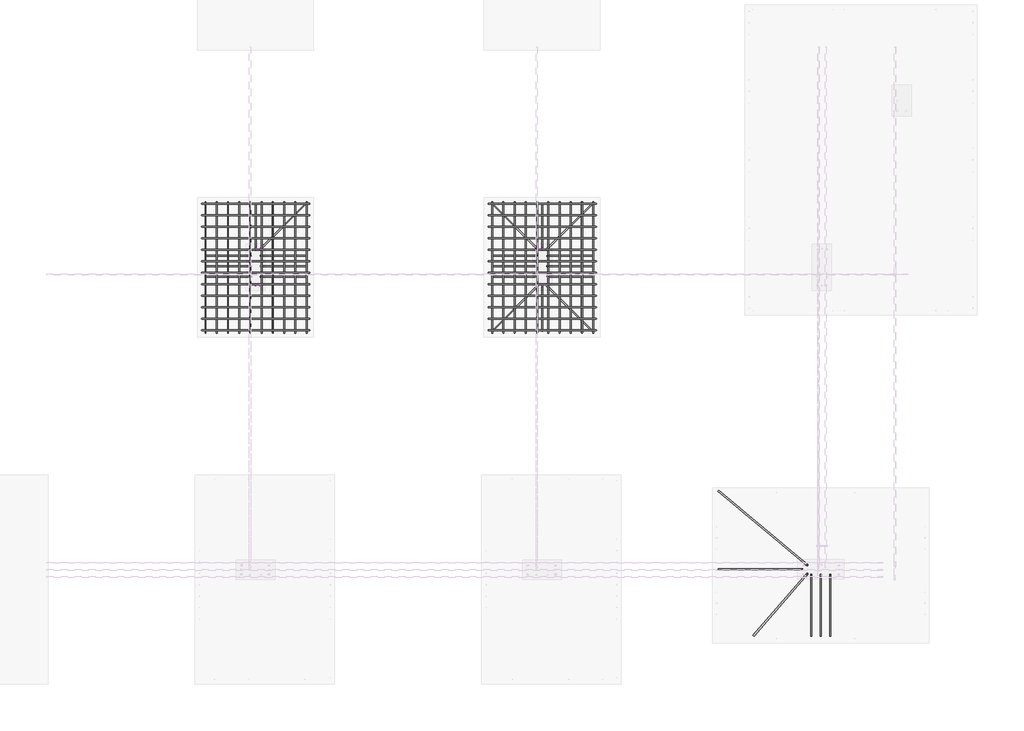
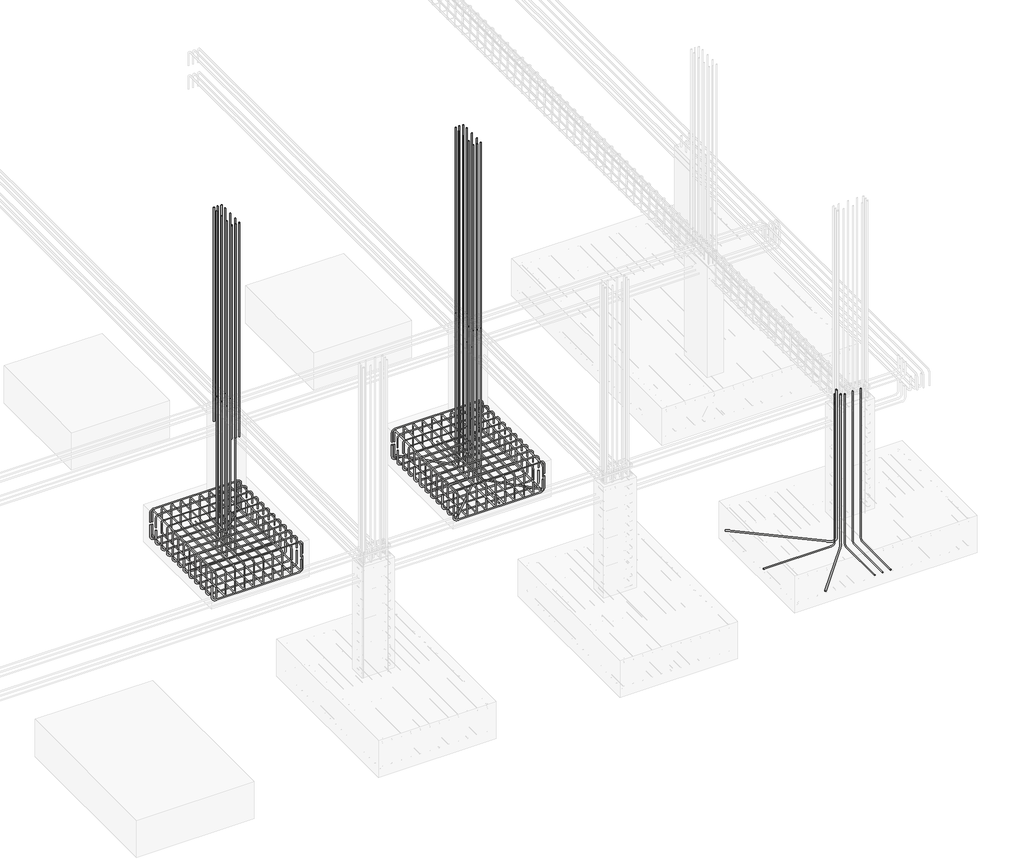
# One storey, part 8 of 18: 40 reinforcing bars.
"""IFC4 building model written with IfcOpenShell, lengths in millimetres."""

from ifc_helpers import new_model, si_unit, point, frame, origin, place, context, project, spatial, polyline, circle_curve, trimmed, segment, composite_curve, source, transform, mapped, element, save
from ifc_brep_helpers import swept_disk

model = new_model("IFC4")

# Units and contexts
model_context = context("Model", 3, world=origin())
ifc_project = project(units=[si_unit("LENGTHUNIT", "METRE", prefix="MILLI")], contexts=[model_context])

# Site, building, storey
site = spatial("IfcSite", under=ifc_project)
building = spatial("IfcBuilding", under=site)
storey = spatial("IfcBuildingStorey", under=building, Elevation=-2000.0)

# Reinforcing bars
placement = place(None, origin())
reinforcing_bar_shape = source(origin(), model_context, "Body", "SolidModel", [
    swept_disk(composite_curve([segment(polyline([(2921.4600308, -834.8555128, -2300.0), (2921.4600308, -834.8555128, -2486.6)]), True, "CONTINUOUS"), segment(trimmed(circle_curve(frame((2866.0100308, -834.8555128, -2486.6), z_axis=(0.0, 1.0, 0.0), x_axis=(55.44999999999982, 0.0, 0.0)), 55.45), [point((2921.4600308, -834.8555128, -2486.6))], [point((2866.0100308, -834.8555128, -2542.05))], True, "CARTESIAN"), True, "CONTINUOUS"), segment(polyline([(2866.0100308, -834.8555128, -2542.05), (1592.8100308, -834.8555128, -2542.05)]), True, "CONTINUOUS"), segment(trimmed(circle_curve(frame((1592.8100308, -834.8555128, -2486.6), z_axis=(0.0, 1.0, 0.0), x_axis=(0.0, 0.0, -55.45000000000027)), 55.45), [point((1592.8100308, -834.8555128, -2542.05))], [point((1537.3600308, -834.8555128, -2486.6))], True, "CARTESIAN"), True, "CONTINUOUS"), segment(polyline([(1537.3600308, -834.8555128, -2486.6), (1537.3600308, -834.8555128, -2300.0)]), True, "CONTINUOUS")], self_intersect=False), 7.95),
])
element("IfcReinforcingBar", 1, at=placement, inside=storey, context=model_context, shape_type="MappedRepresentation", body=[
    mapped(reinforcing_bar_shape, transform((0.0, 0.0, 0.0), x_axis=(1.0, 0.0, 0.0), y_axis=(0.0, 1.0, 0.0), z_axis=(0.0, 0.0, 1.0))),
    mapped(reinforcing_bar_shape, transform((0.0, -148.4250709, 0.0), x_axis=(1.0, 0.0, 0.0), y_axis=(0.0, 1.0, 0.0), z_axis=(0.0, 0.0, 1.0))),
    mapped(reinforcing_bar_shape, transform((0.0, -296.8501418, 0.0), x_axis=(1.0, 0.0, 0.0), y_axis=(0.0, 1.0, 0.0), z_axis=(0.0, 0.0, 1.0))),
    mapped(reinforcing_bar_shape, transform((0.0, -445.2752126, 0.0), x_axis=(1.0, 0.0, 0.0), y_axis=(0.0, 1.0, 0.0), z_axis=(0.0, 0.0, 1.0))),
    mapped(reinforcing_bar_shape, transform((0.0, -593.7002835, 0.0), x_axis=(1.0, 0.0, 0.0), y_axis=(0.0, 1.0, 0.0), z_axis=(0.0, 0.0, 1.0))),
    mapped(reinforcing_bar_shape, transform((0.0, -742.1253544, 0.0), x_axis=(1.0, 0.0, 0.0), y_axis=(0.0, 1.0, 0.0), z_axis=(0.0, 0.0, 1.0))),
    mapped(reinforcing_bar_shape, transform((0.0, -890.5504253, 0.0), x_axis=(1.0, 0.0, 0.0), y_axis=(0.0, 1.0, 0.0), z_axis=(0.0, 0.0, 1.0))),
    mapped(reinforcing_bar_shape, transform((0.0, -1038.9754961, 0.0), x_axis=(1.0, 0.0, 0.0), y_axis=(0.0, 1.0, 0.0), z_axis=(0.0, 0.0, 1.0))),
    mapped(reinforcing_bar_shape, transform((0.0, -1187.400567, 0.0), x_axis=(1.0, 0.0, 0.0), y_axis=(0.0, 1.0, 0.0), z_axis=(0.0, 0.0, 1.0))),
    mapped(reinforcing_bar_shape, transform((0.0, -1335.8256379, 0.0), x_axis=(1.0, 0.0, 0.0), y_axis=(0.0, 1.0, 0.0), z_axis=(0.0, 0.0, 1.0))),
    mapped(reinforcing_bar_shape, transform((0.0, -1484.2507088, 0.0), x_axis=(1.0, 0.0, 0.0), y_axis=(0.0, 1.0, 0.0), z_axis=(0.0, 0.0, 1.0))),
    mapped(reinforcing_bar_shape, transform((0.0, -1632.6757796, 0.0), x_axis=(1.0, 0.0, 0.0), y_axis=(0.0, 1.0, 0.0), z_axis=(0.0, 0.0, 1.0))),
])
reinforcing_bar_2_shape = source(origin(), model_context, "Body", "SolidModel", [
    swept_disk(composite_curve([segment(polyline([(1535.4100308, -834.8555128, -2250.0), (1535.4100308, -834.8555128, -2102.0)]), True, "CONTINUOUS"), segment(trimmed(circle_curve(frame((1581.4100308, -834.8555128, -2102.0), z_axis=(0.0, 1.0, 0.0), x_axis=(-46.0, 0.0, 0.0)), 46.0), [point((1535.4100308, -834.8555128, -2102.0))], [point((1581.4100308, -834.8555128, -2056.0))], True, "CARTESIAN"), True, "CONTINUOUS"), segment(polyline([(1581.4100308, -834.8555128, -2056.0), (2877.4100308, -834.8555128, -2056.0)]), True, "CONTINUOUS"), segment(trimmed(circle_curve(frame((2877.4100308, -834.8555128, -2102.0), z_axis=(0.0, 1.0, 0.0), x_axis=(0.0, 0.0, 46.0)), 46.0), [point((2877.4100308, -834.8555128, -2056.0))], [point((2923.4100308, -834.8555128, -2102.0))], True, "CARTESIAN"), True, "CONTINUOUS"), segment(polyline([(2923.4100308, -834.8555128, -2102.0), (2923.4100308, -834.8555128, -2250.0)]), True, "CONTINUOUS")], self_intersect=False), 6.0),
])
element("IfcReinforcingBar", 2, at=placement, inside=storey, context=model_context, shape_type="MappedRepresentation", body=[
    mapped(reinforcing_bar_2_shape, transform((0.0, 0.0, 0.0), x_axis=(1.0, 0.0, 0.0), y_axis=(0.0, 1.0, 0.0), z_axis=(0.0, 0.0, 1.0))),
    mapped(reinforcing_bar_2_shape, transform((0.0, -148.4250709, 0.0), x_axis=(1.0, 0.0, 0.0), y_axis=(0.0, 1.0, 0.0), z_axis=(0.0, 0.0, 1.0))),
    mapped(reinforcing_bar_2_shape, transform((0.0, -296.8501418, 0.0), x_axis=(1.0, 0.0, 0.0), y_axis=(0.0, 1.0, 0.0), z_axis=(0.0, 0.0, 1.0))),
    mapped(reinforcing_bar_2_shape, transform((0.0, -445.2752126, 0.0), x_axis=(1.0, 0.0, 0.0), y_axis=(0.0, 1.0, 0.0), z_axis=(0.0, 0.0, 1.0))),
    mapped(reinforcing_bar_2_shape, transform((0.0, -593.7002835, 0.0), x_axis=(1.0, 0.0, 0.0), y_axis=(0.0, 1.0, 0.0), z_axis=(0.0, 0.0, 1.0))),
    mapped(reinforcing_bar_2_shape, transform((0.0, -742.1253544, 0.0), x_axis=(1.0, 0.0, 0.0), y_axis=(0.0, 1.0, 0.0), z_axis=(0.0, 0.0, 1.0))),
    mapped(reinforcing_bar_2_shape, transform((0.0, -890.5504253, 0.0), x_axis=(1.0, 0.0, 0.0), y_axis=(0.0, 1.0, 0.0), z_axis=(0.0, 0.0, 1.0))),
    mapped(reinforcing_bar_2_shape, transform((0.0, -1038.9754961, 0.0), x_axis=(1.0, 0.0, 0.0), y_axis=(0.0, 1.0, 0.0), z_axis=(0.0, 0.0, 1.0))),
    mapped(reinforcing_bar_2_shape, transform((0.0, -1187.400567, 0.0), x_axis=(1.0, 0.0, 0.0), y_axis=(0.0, 1.0, 0.0), z_axis=(0.0, 0.0, 1.0))),
    mapped(reinforcing_bar_2_shape, transform((0.0, -1335.8256379, 0.0), x_axis=(1.0, 0.0, 0.0), y_axis=(0.0, 1.0, 0.0), z_axis=(0.0, 0.0, 1.0))),
    mapped(reinforcing_bar_2_shape, transform((0.0, -1484.2507088, 0.0), x_axis=(1.0, 0.0, 0.0), y_axis=(0.0, 1.0, 0.0), z_axis=(0.0, 0.0, 1.0))),
    mapped(reinforcing_bar_2_shape, transform((0.0, -1632.6757796, 0.0), x_axis=(1.0, 0.0, 0.0), y_axis=(0.0, 1.0, 0.0), z_axis=(0.0, 0.0, 1.0))),
])
reinforcing_bar_3_shape = source(origin(), model_context, "Body", "SolidModel", [
    swept_disk(composite_curve([segment(polyline([(1581.5908136, -811.9600376, -2322.6684255), (1581.5908136, -811.9600376, -2470.6684255)]), True, "CONTINUOUS"), segment(trimmed(circle_curve(frame((1581.5908136, -857.9600376, -2470.6684255), z_axis=(-1.0, 0.0, 0.0), x_axis=(0.0, 46.0, 0.0)), 46.0), [point((1581.5908136, -811.9600376, -2470.6684255))], [point((1581.5908136, -857.9600376, -2516.6684255))], True, "CARTESIAN"), True, "CONTINUOUS"), segment(polyline([(1581.5908136, -857.9600376, -2516.6684255), (1581.5908136, -2453.9600376, -2516.6684255)]), True, "CONTINUOUS"), segment(trimmed(circle_curve(frame((1581.5908136, -2453.9600376, -2470.6684255), z_axis=(-1.0, 0.0, 0.0), x_axis=(0.0, 0.0, -46.0)), 46.0), [point((1581.5908136, -2453.9600376, -2516.6684255))], [point((1581.5908136, -2499.9600376, -2470.6684255))], True, "CARTESIAN"), True, "CONTINUOUS"), segment(polyline([(1581.5908136, -2499.9600376, -2470.6684255), (1581.5908136, -2499.9600376, -2322.6684255)]), True, "CONTINUOUS")], self_intersect=False), 6.0),
])
element("IfcReinforcingBar", 3, at=placement, inside=storey, context=model_context, shape_type="MappedRepresentation", body=[
    mapped(reinforcing_bar_3_shape, transform((0.0, 0.0, 0.0), x_axis=(1.0, 0.0, 0.0), y_axis=(0.0, 1.0, 0.0), z_axis=(0.0, 0.0, 1.0))),
    mapped(reinforcing_bar_3_shape, transform((144.8687847, 0.0, 0.0), x_axis=(1.0, 0.0, 0.0), y_axis=(0.0, 1.0, 0.0), z_axis=(0.0, 0.0, 1.0))),
    mapped(reinforcing_bar_3_shape, transform((289.7375694, 0.0, 0.0), x_axis=(1.0, 0.0, 0.0), y_axis=(0.0, 1.0, 0.0), z_axis=(0.0, 0.0, 1.0))),
    mapped(reinforcing_bar_3_shape, transform((434.6063541, 0.0, 0.0), x_axis=(1.0, 0.0, 0.0), y_axis=(0.0, 1.0, 0.0), z_axis=(0.0, 0.0, 1.0))),
    mapped(reinforcing_bar_3_shape, transform((579.4751388, 0.0, 0.0), x_axis=(1.0, 0.0, 0.0), y_axis=(0.0, 1.0, 0.0), z_axis=(0.0, 0.0, 1.0))),
    mapped(reinforcing_bar_3_shape, transform((724.3439235, 0.0, 0.0), x_axis=(1.0, 0.0, 0.0), y_axis=(0.0, 1.0, 0.0), z_axis=(0.0, 0.0, 1.0))),
    mapped(reinforcing_bar_3_shape, transform((869.2127082, 0.0, 0.0), x_axis=(1.0, 0.0, 0.0), y_axis=(0.0, 1.0, 0.0), z_axis=(0.0, 0.0, 1.0))),
    mapped(reinforcing_bar_3_shape, transform((1014.0814929, 0.0, 0.0), x_axis=(1.0, 0.0, 0.0), y_axis=(0.0, 1.0, 0.0), z_axis=(0.0, 0.0, 1.0))),
    mapped(reinforcing_bar_3_shape, transform((1158.9502776, 0.0, 0.0), x_axis=(1.0, 0.0, 0.0), y_axis=(0.0, 1.0, 0.0), z_axis=(0.0, 0.0, 1.0))),
    mapped(reinforcing_bar_3_shape, transform((1303.8190623, 0.0, 0.0), x_axis=(1.0, 0.0, 0.0), y_axis=(0.0, 1.0, 0.0), z_axis=(0.0, 0.0, 1.0))),
])
reinforcing_bar_4_shape = source(origin(), model_context, "Body", "SolidModel", [
    swept_disk(composite_curve([segment(polyline([(2887.3330478, -811.9600376, -2276.6677805), (2887.3330478, -811.9600376, -2128.6677805)]), True, "CONTINUOUS"), segment(trimmed(circle_curve(frame((2887.3330478, -857.9600376, -2128.6677805), z_axis=(1.0, 0.0, 0.0), x_axis=(0.0, 46.0, 0.0)), 46.0), [point((2887.3330478, -811.9600376, -2128.6677805))], [point((2887.3330478, -857.9600376, -2082.6677805))], True, "CARTESIAN"), True, "CONTINUOUS"), segment(polyline([(2887.3330478, -857.9600376, -2082.6677805), (2887.3330478, -2453.9600376, -2082.6677805)]), True, "CONTINUOUS"), segment(trimmed(circle_curve(frame((2887.3330478, -2453.9600376, -2128.6677805), z_axis=(1.0, 0.0, 0.0), x_axis=(0.0, 0.0, 46.0)), 46.0), [point((2887.3330478, -2453.9600376, -2082.6677805))], [point((2887.3330478, -2499.9600376, -2128.6677805))], True, "CARTESIAN"), True, "CONTINUOUS"), segment(polyline([(2887.3330478, -2499.9600376, -2128.6677805), (2887.3330478, -2499.9600376, -2276.6677805)]), True, "CONTINUOUS")], self_intersect=False), 6.0),
])
element("IfcReinforcingBar", 4, at=placement, inside=storey, context=model_context, shape_type="MappedRepresentation", body=[
    mapped(reinforcing_bar_4_shape, transform((0.0, 0.0, 0.0), x_axis=(1.0, 0.0, 0.0), y_axis=(0.0, 1.0, 0.0), z_axis=(0.0, 0.0, 1.0))),
    mapped(reinforcing_bar_4_shape, transform((-145.0824705, 0.0, 0.0), x_axis=(1.0, 0.0, 0.0), y_axis=(0.0, 1.0, 0.0), z_axis=(0.0, 0.0, 1.0))),
    mapped(reinforcing_bar_4_shape, transform((-290.1649409, 0.0, 0.0), x_axis=(1.0, 0.0, 0.0), y_axis=(0.0, 1.0, 0.0), z_axis=(0.0, 0.0, 1.0))),
    mapped(reinforcing_bar_4_shape, transform((-435.2474114, 0.0, 0.0), x_axis=(1.0, 0.0, 0.0), y_axis=(0.0, 1.0, 0.0), z_axis=(0.0, 0.0, 1.0))),
    mapped(reinforcing_bar_4_shape, transform((-580.3298819, 0.0, 0.0), x_axis=(1.0, 0.0, 0.0), y_axis=(0.0, 1.0, 0.0), z_axis=(0.0, 0.0, 1.0))),
    mapped(reinforcing_bar_4_shape, transform((-725.4123523, 0.0, 0.0), x_axis=(1.0, 0.0, 0.0), y_axis=(0.0, 1.0, 0.0), z_axis=(0.0, 0.0, 1.0))),
    mapped(reinforcing_bar_4_shape, transform((-870.4948228, 0.0, 0.0), x_axis=(1.0, 0.0, 0.0), y_axis=(0.0, 1.0, 0.0), z_axis=(0.0, 0.0, 1.0))),
    mapped(reinforcing_bar_4_shape, transform((-1015.5772932, 0.0, 0.0), x_axis=(1.0, 0.0, 0.0), y_axis=(0.0, 1.0, 0.0), z_axis=(0.0, 0.0, 1.0))),
    mapped(reinforcing_bar_4_shape, transform((-1160.6597637, 0.0, 0.0), x_axis=(1.0, 0.0, 0.0), y_axis=(0.0, 1.0, 0.0), z_axis=(0.0, 0.0, 1.0))),
    mapped(reinforcing_bar_4_shape, transform((-1305.7422342, 0.0, 0.0), x_axis=(1.0, 0.0, 0.0), y_axis=(0.0, 1.0, 0.0), z_axis=(0.0, 0.0, 1.0))),
])
reinforcing_bar_5_shape = source(origin(), model_context, "Body", "SolidModel", [
    swept_disk(composite_curve([segment(polyline([(6621.4600308, -834.8555128, -2300.0), (6621.4600308, -834.8555128, -2486.6)]), True, "CONTINUOUS"), segment(trimmed(circle_curve(frame((6566.0100308, -834.8555128, -2486.6), z_axis=(0.0, 1.0, 0.0), x_axis=(55.44999999999982, 0.0, 0.0)), 55.45), [point((6621.4600308, -834.8555128, -2486.6))], [point((6566.0100308, -834.8555128, -2542.05))], True, "CARTESIAN"), True, "CONTINUOUS"), segment(polyline([(6566.0100308, -834.8555128, -2542.05), (5292.8100308, -834.8555128, -2542.05)]), True, "CONTINUOUS"), segment(trimmed(circle_curve(frame((5292.8100308, -834.8555128, -2486.6), z_axis=(0.0, 1.0, 0.0), x_axis=(0.0, 0.0, -55.45000000000027)), 55.45), [point((5292.8100308, -834.8555128, -2542.05))], [point((5237.3600308, -834.8555128, -2486.6))], True, "CARTESIAN"), True, "CONTINUOUS"), segment(polyline([(5237.3600308, -834.8555128, -2486.6), (5237.3600308, -834.8555128, -2300.0)]), True, "CONTINUOUS")], self_intersect=False), 7.95),
])
element("IfcReinforcingBar", 5, at=placement, inside=storey, context=model_context, shape_type="MappedRepresentation", body=[
    mapped(reinforcing_bar_5_shape, transform((0.0, 0.0, 0.0), x_axis=(1.0, 0.0, 0.0), y_axis=(0.0, 1.0, 0.0), z_axis=(0.0, 0.0, 1.0))),
    mapped(reinforcing_bar_5_shape, transform((0.0, -148.4250709, 0.0), x_axis=(1.0, 0.0, 0.0), y_axis=(0.0, 1.0, 0.0), z_axis=(0.0, 0.0, 1.0))),
    mapped(reinforcing_bar_5_shape, transform((0.0, -296.8501418, 0.0), x_axis=(1.0, 0.0, 0.0), y_axis=(0.0, 1.0, 0.0), z_axis=(0.0, 0.0, 1.0))),
    mapped(reinforcing_bar_5_shape, transform((0.0, -445.2752126, 0.0), x_axis=(1.0, 0.0, 0.0), y_axis=(0.0, 1.0, 0.0), z_axis=(0.0, 0.0, 1.0))),
    mapped(reinforcing_bar_5_shape, transform((0.0, -593.7002835, 0.0), x_axis=(1.0, 0.0, 0.0), y_axis=(0.0, 1.0, 0.0), z_axis=(0.0, 0.0, 1.0))),
    mapped(reinforcing_bar_5_shape, transform((0.0, -742.1253544, 0.0), x_axis=(1.0, 0.0, 0.0), y_axis=(0.0, 1.0, 0.0), z_axis=(0.0, 0.0, 1.0))),
    mapped(reinforcing_bar_5_shape, transform((0.0, -890.5504253, 0.0), x_axis=(1.0, 0.0, 0.0), y_axis=(0.0, 1.0, 0.0), z_axis=(0.0, 0.0, 1.0))),
    mapped(reinforcing_bar_5_shape, transform((0.0, -1038.9754961, 0.0), x_axis=(1.0, 0.0, 0.0), y_axis=(0.0, 1.0, 0.0), z_axis=(0.0, 0.0, 1.0))),
    mapped(reinforcing_bar_5_shape, transform((0.0, -1187.400567, 0.0), x_axis=(1.0, 0.0, 0.0), y_axis=(0.0, 1.0, 0.0), z_axis=(0.0, 0.0, 1.0))),
    mapped(reinforcing_bar_5_shape, transform((0.0, -1335.8256379, 0.0), x_axis=(1.0, 0.0, 0.0), y_axis=(0.0, 1.0, 0.0), z_axis=(0.0, 0.0, 1.0))),
    mapped(reinforcing_bar_5_shape, transform((0.0, -1484.2507088, 0.0), x_axis=(1.0, 0.0, 0.0), y_axis=(0.0, 1.0, 0.0), z_axis=(0.0, 0.0, 1.0))),
    mapped(reinforcing_bar_5_shape, transform((0.0, -1632.6757796, 0.0), x_axis=(1.0, 0.0, 0.0), y_axis=(0.0, 1.0, 0.0), z_axis=(0.0, 0.0, 1.0))),
])
reinforcing_bar_6_shape = source(origin(), model_context, "Body", "SolidModel", [
    swept_disk(composite_curve([segment(polyline([(5235.4100308, -834.8555128, -2250.0), (5235.4100308, -834.8555128, -2102.0)]), True, "CONTINUOUS"), segment(trimmed(circle_curve(frame((5281.4100308, -834.8555128, -2102.0), z_axis=(0.0, 1.0, 0.0), x_axis=(-46.0, 0.0, 0.0)), 46.0), [point((5235.4100308, -834.8555128, -2102.0))], [point((5281.4100308, -834.8555128, -2056.0))], True, "CARTESIAN"), True, "CONTINUOUS"), segment(polyline([(5281.4100308, -834.8555128, -2056.0), (6577.4100308, -834.8555128, -2056.0)]), True, "CONTINUOUS"), segment(trimmed(circle_curve(frame((6577.4100308, -834.8555128, -2102.0), z_axis=(0.0, 1.0, 0.0), x_axis=(0.0, 0.0, 46.0)), 46.0), [point((6577.4100308, -834.8555128, -2056.0))], [point((6623.4100308, -834.8555128, -2102.0))], True, "CARTESIAN"), True, "CONTINUOUS"), segment(polyline([(6623.4100308, -834.8555128, -2102.0), (6623.4100308, -834.8555128, -2250.0)]), True, "CONTINUOUS")], self_intersect=False), 6.0),
])
element("IfcReinforcingBar", 6, at=placement, inside=storey, context=model_context, shape_type="MappedRepresentation", body=[
    mapped(reinforcing_bar_6_shape, transform((0.0, 0.0, 0.0), x_axis=(1.0, 0.0, 0.0), y_axis=(0.0, 1.0, 0.0), z_axis=(0.0, 0.0, 1.0))),
    mapped(reinforcing_bar_6_shape, transform((0.0, -148.4250709, 0.0), x_axis=(1.0, 0.0, 0.0), y_axis=(0.0, 1.0, 0.0), z_axis=(0.0, 0.0, 1.0))),
    mapped(reinforcing_bar_6_shape, transform((0.0, -296.8501418, 0.0), x_axis=(1.0, 0.0, 0.0), y_axis=(0.0, 1.0, 0.0), z_axis=(0.0, 0.0, 1.0))),
    mapped(reinforcing_bar_6_shape, transform((0.0, -445.2752126, 0.0), x_axis=(1.0, 0.0, 0.0), y_axis=(0.0, 1.0, 0.0), z_axis=(0.0, 0.0, 1.0))),
    mapped(reinforcing_bar_6_shape, transform((0.0, -593.7002835, 0.0), x_axis=(1.0, 0.0, 0.0), y_axis=(0.0, 1.0, 0.0), z_axis=(0.0, 0.0, 1.0))),
    mapped(reinforcing_bar_6_shape, transform((0.0, -742.1253544, 0.0), x_axis=(1.0, 0.0, 0.0), y_axis=(0.0, 1.0, 0.0), z_axis=(0.0, 0.0, 1.0))),
    mapped(reinforcing_bar_6_shape, transform((0.0, -890.5504253, 0.0), x_axis=(1.0, 0.0, 0.0), y_axis=(0.0, 1.0, 0.0), z_axis=(0.0, 0.0, 1.0))),
    mapped(reinforcing_bar_6_shape, transform((0.0, -1038.9754961, 0.0), x_axis=(1.0, 0.0, 0.0), y_axis=(0.0, 1.0, 0.0), z_axis=(0.0, 0.0, 1.0))),
    mapped(reinforcing_bar_6_shape, transform((0.0, -1187.400567, 0.0), x_axis=(1.0, 0.0, 0.0), y_axis=(0.0, 1.0, 0.0), z_axis=(0.0, 0.0, 1.0))),
    mapped(reinforcing_bar_6_shape, transform((0.0, -1335.8256379, 0.0), x_axis=(1.0, 0.0, 0.0), y_axis=(0.0, 1.0, 0.0), z_axis=(0.0, 0.0, 1.0))),
    mapped(reinforcing_bar_6_shape, transform((0.0, -1484.2507088, 0.0), x_axis=(1.0, 0.0, 0.0), y_axis=(0.0, 1.0, 0.0), z_axis=(0.0, 0.0, 1.0))),
    mapped(reinforcing_bar_6_shape, transform((0.0, -1632.6757796, 0.0), x_axis=(1.0, 0.0, 0.0), y_axis=(0.0, 1.0, 0.0), z_axis=(0.0, 0.0, 1.0))),
])
reinforcing_bar_7_shape = source(origin(), model_context, "Body", "SolidModel", [
    swept_disk(composite_curve([segment(polyline([(5281.5908136, -811.9600376, -2322.6684255), (5281.5908136, -811.9600376, -2470.6684255)]), True, "CONTINUOUS"), segment(trimmed(circle_curve(frame((5281.5908136, -857.9600376, -2470.6684255), z_axis=(-1.0, 0.0, 0.0), x_axis=(0.0, 46.0, 0.0)), 46.0), [point((5281.5908136, -811.9600376, -2470.6684255))], [point((5281.5908136, -857.9600376, -2516.6684255))], True, "CARTESIAN"), True, "CONTINUOUS"), segment(polyline([(5281.5908136, -857.9600376, -2516.6684255), (5281.5908136, -2453.9600376, -2516.6684255)]), True, "CONTINUOUS"), segment(trimmed(circle_curve(frame((5281.5908136, -2453.9600376, -2470.6684255), z_axis=(-1.0, 0.0, 0.0), x_axis=(0.0, 0.0, -46.0)), 46.0), [point((5281.5908136, -2453.9600376, -2516.6684255))], [point((5281.5908136, -2499.9600376, -2470.6684255))], True, "CARTESIAN"), True, "CONTINUOUS"), segment(polyline([(5281.5908136, -2499.9600376, -2470.6684255), (5281.5908136, -2499.9600376, -2322.6684255)]), True, "CONTINUOUS")], self_intersect=False), 6.0),
])
element("IfcReinforcingBar", 7, at=placement, inside=storey, context=model_context, shape_type="MappedRepresentation", body=[
    mapped(reinforcing_bar_7_shape, transform((0.0, 0.0, 0.0), x_axis=(1.0, 0.0, 0.0), y_axis=(0.0, 1.0, 0.0), z_axis=(0.0, 0.0, 1.0))),
    mapped(reinforcing_bar_7_shape, transform((144.8687847, 0.0, 0.0), x_axis=(1.0, 0.0, 0.0), y_axis=(0.0, 1.0, 0.0), z_axis=(0.0, 0.0, 1.0))),
    mapped(reinforcing_bar_7_shape, transform((289.7375694, 0.0, 0.0), x_axis=(1.0, 0.0, 0.0), y_axis=(0.0, 1.0, 0.0), z_axis=(0.0, 0.0, 1.0))),
    mapped(reinforcing_bar_7_shape, transform((434.6063541, 0.0, 0.0), x_axis=(1.0, 0.0, 0.0), y_axis=(0.0, 1.0, 0.0), z_axis=(0.0, 0.0, 1.0))),
    mapped(reinforcing_bar_7_shape, transform((579.4751388, 0.0, 0.0), x_axis=(1.0, 0.0, 0.0), y_axis=(0.0, 1.0, 0.0), z_axis=(0.0, 0.0, 1.0))),
    mapped(reinforcing_bar_7_shape, transform((724.3439235, 0.0, 0.0), x_axis=(1.0, 0.0, 0.0), y_axis=(0.0, 1.0, 0.0), z_axis=(0.0, 0.0, 1.0))),
    mapped(reinforcing_bar_7_shape, transform((869.2127082, 0.0, 0.0), x_axis=(1.0, 0.0, 0.0), y_axis=(0.0, 1.0, 0.0), z_axis=(0.0, 0.0, 1.0))),
    mapped(reinforcing_bar_7_shape, transform((1014.0814929, 0.0, 0.0), x_axis=(1.0, 0.0, 0.0), y_axis=(0.0, 1.0, 0.0), z_axis=(0.0, 0.0, 1.0))),
    mapped(reinforcing_bar_7_shape, transform((1158.9502776, 0.0, 0.0), x_axis=(1.0, 0.0, 0.0), y_axis=(0.0, 1.0, 0.0), z_axis=(0.0, 0.0, 1.0))),
    mapped(reinforcing_bar_7_shape, transform((1303.8190623, 0.0, 0.0), x_axis=(1.0, 0.0, 0.0), y_axis=(0.0, 1.0, 0.0), z_axis=(0.0, 0.0, 1.0))),
])
reinforcing_bar_8_shape = source(origin(), model_context, "Body", "SolidModel", [
    swept_disk(composite_curve([segment(polyline([(6587.3330478, -811.9600376, -2276.6677805), (6587.3330478, -811.9600376, -2128.6677805)]), True, "CONTINUOUS"), segment(trimmed(circle_curve(frame((6587.3330478, -857.9600376, -2128.6677805), z_axis=(1.0, 0.0, 0.0), x_axis=(0.0, 46.0, 0.0)), 46.0), [point((6587.3330478, -811.9600376, -2128.6677805))], [point((6587.3330478, -857.9600376, -2082.6677805))], True, "CARTESIAN"), True, "CONTINUOUS"), segment(polyline([(6587.3330478, -857.9600376, -2082.6677805), (6587.3330478, -2453.9600376, -2082.6677805)]), True, "CONTINUOUS"), segment(trimmed(circle_curve(frame((6587.3330478, -2453.9600376, -2128.6677805), z_axis=(1.0, 0.0, 0.0), x_axis=(0.0, 0.0, 46.0)), 46.0), [point((6587.3330478, -2453.9600376, -2082.6677805))], [point((6587.3330478, -2499.9600376, -2128.6677805))], True, "CARTESIAN"), True, "CONTINUOUS"), segment(polyline([(6587.3330478, -2499.9600376, -2128.6677805), (6587.3330478, -2499.9600376, -2276.6677805)]), True, "CONTINUOUS")], self_intersect=False), 6.0),
])
element("IfcReinforcingBar", 8, at=placement, inside=storey, context=model_context, shape_type="MappedRepresentation", body=[
    mapped(reinforcing_bar_8_shape, transform((0.0, 0.0, 0.0), x_axis=(1.0, 0.0, 0.0), y_axis=(0.0, 1.0, 0.0), z_axis=(0.0, 0.0, 1.0))),
    mapped(reinforcing_bar_8_shape, transform((-145.0824705, 0.0, 0.0), x_axis=(1.0, 0.0, 0.0), y_axis=(0.0, 1.0, 0.0), z_axis=(0.0, 0.0, 1.0))),
    mapped(reinforcing_bar_8_shape, transform((-290.1649409, 0.0, 0.0), x_axis=(1.0, 0.0, 0.0), y_axis=(0.0, 1.0, 0.0), z_axis=(0.0, 0.0, 1.0))),
    mapped(reinforcing_bar_8_shape, transform((-435.2474114, 0.0, 0.0), x_axis=(1.0, 0.0, 0.0), y_axis=(0.0, 1.0, 0.0), z_axis=(0.0, 0.0, 1.0))),
    mapped(reinforcing_bar_8_shape, transform((-580.3298819, 0.0, 0.0), x_axis=(1.0, 0.0, 0.0), y_axis=(0.0, 1.0, 0.0), z_axis=(0.0, 0.0, 1.0))),
    mapped(reinforcing_bar_8_shape, transform((-725.4123523, 0.0, 0.0), x_axis=(1.0, 0.0, 0.0), y_axis=(0.0, 1.0, 0.0), z_axis=(0.0, 0.0, 1.0))),
    mapped(reinforcing_bar_8_shape, transform((-870.4948228, 0.0, 0.0), x_axis=(1.0, 0.0, 0.0), y_axis=(0.0, 1.0, 0.0), z_axis=(0.0, 0.0, 1.0))),
    mapped(reinforcing_bar_8_shape, transform((-1015.5772932, 0.0, 0.0), x_axis=(1.0, 0.0, 0.0), y_axis=(0.0, 1.0, 0.0), z_axis=(0.0, 0.0, 1.0))),
    mapped(reinforcing_bar_8_shape, transform((-1160.6597637, 0.0, 0.0), x_axis=(1.0, 0.0, 0.0), y_axis=(0.0, 1.0, 0.0), z_axis=(0.0, 0.0, 1.0))),
    mapped(reinforcing_bar_8_shape, transform((-1305.7422342, 0.0, 0.0), x_axis=(1.0, 0.0, 0.0), y_axis=(0.0, 1.0, 0.0), z_axis=(0.0, 0.0, 1.0))),
])
element("IfcReinforcingBar", 9, at=placement, inside=storey, context=model_context, shape_type="SolidModel", body=[
    swept_disk(composite_curve([segment(polyline([(8202.5916138, -4537.960597, -2480.0), (9296.0051153, -5455.4434628, -2480.0)]), True, "CONTINUOUS"), segment(trimmed(circle_curve(frame((9296.0051153, -5455.4434628, -2412.5), z_axis=(-0.6427876096865429, -0.766044443118975, 0.0), x_axis=(0.0, 0.0, -67.5)), 67.5), [point((9296.0051153, -5455.4434628, -2480.0))], [point((9347.7131152, -5498.8316264, -2412.5))], True, "CARTESIAN"), True, "CONTINUOUS"), segment(polyline([(9347.7131152, -5498.8316264, -2412.5), (9347.7131152, -5498.8316264, -20.0)]), True, "CONTINUOUS")], self_intersect=False), 10.0),
])
element("IfcReinforcingBar", 10, at=placement, inside=storey, context=model_context, shape_type="SolidModel", body=[
    swept_disk(composite_curve([segment(polyline([(8198.5572946, -5554.0856321, -2480.0), (9241.3529891, -5554.0856321, -2480.0)]), True, "CONTINUOUS"), segment(trimmed(circle_curve(frame((9241.3529891, -5554.0856321, -2434.0), z_axis=(0.0, -1.0, 0.0), x_axis=(0.0, 0.0, -46.0)), 46.0), [point((9241.3529891, -5554.0856321, -2480.0))], [point((9287.3529891, -5554.0856321, -2434.0))], True, "CARTESIAN"), True, "CONTINUOUS"), segment(polyline([(9287.3529891, -5554.0856321, -2434.0), (9287.3529891, -5554.0856321, -30.0)]), True, "CONTINUOUS")], self_intersect=False), 6.0),
])
element("IfcReinforcingBar", 11, at=placement, inside=storey, context=model_context, shape_type="SolidModel", body=[
    swept_disk(composite_curve([segment(polyline([(8655.8433207, -6409.8777562, -2480.0), (9303.4291308, -5664.9154994, -2480.0)]), True, "CONTINUOUS"), segment(trimmed(circle_curve(frame((9303.4291308, -5664.9154994, -2412.5), z_axis=(0.7547095802227678, -0.6560590289905122, 0.0), x_axis=(0.0, 0.0, -67.5)), 67.5), [point((9303.4291308, -5664.9154994, -2480.0))], [point((9347.7131152, -5613.9726027, -2412.5))], True, "CARTESIAN"), True, "CONTINUOUS"), segment(polyline([(9347.7131152, -5613.9726027, -2412.5), (9347.7131152, -5613.9726027, -20.0)]), True, "CONTINUOUS")], self_intersect=False), 10.0),
])
reinforcing_bar_9_shape = source(origin(), model_context, "Body", "SolidModel", [
    swept_disk(composite_curve([segment(polyline([(9402.8188559, -6417.9733694, -2480.0), (9402.8188559, -5668.4399471, -2480.0)]), True, "CONTINUOUS"), segment(trimmed(circle_curve(frame((9402.8188559, -5668.4399471, -2434.0), z_axis=(1.0, 0.0, 0.0), x_axis=(0.0, 0.0, -46.0)), 46.0), [point((9402.8188559, -5668.4399471, -2480.0))], [point((9402.8188559, -5622.4399471, -2434.0))], True, "CARTESIAN"), True, "CONTINUOUS"), segment(polyline([(9402.8188559, -5622.4399471, -2434.0), (9402.8188559, -5622.4399471, -30.0)]), True, "CONTINUOUS")], self_intersect=False), 6.0),
])
element("IfcReinforcingBar", 12, at=placement, inside=storey, context=model_context, shape_type="MappedRepresentation", body=[
    mapped(reinforcing_bar_9_shape, transform((0.0, 0.0, 0.0), x_axis=(1.0, 0.0, 0.0), y_axis=(0.0, 1.0, 0.0), z_axis=(0.0, 0.0, 1.0))),
    mapped(reinforcing_bar_9_shape, transform((122.4797009, 0.0, 0.0), x_axis=(1.0, 0.0, 0.0), y_axis=(0.0, 1.0, 0.0), z_axis=(0.0, 0.0, 1.0))),
    mapped(reinforcing_bar_9_shape, transform((244.9594019, 0.0, 0.0), x_axis=(1.0, 0.0, 0.0), y_axis=(0.0, 1.0, 0.0), z_axis=(0.0, 0.0, 1.0))),
])
element("IfcReinforcingBar", 13, at=placement, inside=storey, context=model_context, shape_type="SolidModel", body=[
    swept_disk(composite_curve([segment(polyline([(5871.6640946, -1423.0839981, -30.0), (5871.6640946, -1423.0839981, -2431.15)]), True, "CONTINUOUS"), segment(trimmed(circle_curve(frame((5832.4550236, -1383.874927, -2431.15), z_axis=(0.70710678118655, 0.707106781186545, 0.0), x_axis=(39.20907100000022, -39.209071099999846, 0.0)), 55.45), [point((5871.6640946, -1423.0839981, -2431.15))], [point((5832.4550236, -1383.874927, -2486.6))], True, "CARTESIAN"), True, "CONTINUOUS"), segment(polyline([(5832.4550236, -1383.874927, -2486.6), (5286.60971, -838.0296134, -2486.6)]), True, "CONTINUOUS")], self_intersect=False), 7.95),
])
element("IfcReinforcingBar", 14, at=placement, inside=storey, context=model_context, shape_type="SolidModel", body=[
    swept_disk(composite_curve([segment(polyline([(5928.962113, -1418.4824597, -30.0), (5928.962113, -1418.4824597, -2440.6)]), True, "CONTINUOUS"), segment(trimmed(circle_curve(frame((5928.962113, -1372.4824597, -2440.6), z_axis=(1.0, 0.0, 0.0), x_axis=(0.0, -46.0, 0.0)), 46.0), [point((5928.962113, -1418.4824597, -2440.6))], [point((5928.962113, -1372.4824597, -2486.6))], True, "CARTESIAN"), True, "CONTINUOUS"), segment(polyline([(5928.962113, -1372.4824597, -2486.6), (5928.962113, -834.8555128, -2486.6)]), True, "CONTINUOUS")], self_intersect=False), 6.0),
])
reinforcing_bar_10_shape = source(origin(), model_context, "Body", "SolidModel", [
    swept_disk(composite_curve([segment(polyline([(5865.503375, -1776.5422299, -30.0), (5865.503375, -1776.5422299, -2436.6982733)]), True, "CONTINUOUS"), segment(trimmed(circle_curve(frame((5819.503375, -1776.5422299, -2436.6982733), z_axis=(0.0, 1.0, 0.0), x_axis=(46.0, 0.0, 0.0)), 46.0), [point((5865.503375, -1776.5422299, -2436.6982733))], [point((5819.503375, -1776.5422299, -2482.6982733))], True, "CARTESIAN"), True, "CONTINUOUS"), segment(polyline([(5819.503375, -1776.5422299, -2482.6982733), (5282.2732024, -1776.5422299, -2482.6982733)]), True, "CONTINUOUS")], self_intersect=False), 6.0),
])
element("IfcReinforcingBar", 15, at=placement, inside=storey, context=model_context, shape_type="MappedRepresentation", body=[
    mapped(reinforcing_bar_10_shape, transform((0.0, 0.0, 0.0), x_axis=(1.0, 0.0, 0.0), y_axis=(0.0, 1.0, 0.0), z_axis=(0.0, 0.0, 1.0))),
    mapped(reinforcing_bar_10_shape, transform((0.0, 134.2724138, 0.0), x_axis=(1.0, 0.0, 0.0), y_axis=(0.0, 1.0, 0.0), z_axis=(0.0, 0.0, 1.0))),
    mapped(reinforcing_bar_10_shape, transform((0.0, 268.5448277, 0.0), x_axis=(1.0, 0.0, 0.0), y_axis=(0.0, 1.0, 0.0), z_axis=(0.0, 0.0, 1.0))),
])
reinforcing_bar_11_shape = source(origin(), model_context, "Body", "SolidModel", [
    swept_disk(composite_curve([segment(polyline([(5993.3166865, -1776.5422299, -30.0), (5993.3166865, -1776.5422299, -2436.6982733)]), True, "CONTINUOUS"), segment(trimmed(circle_curve(frame((6039.3166865, -1776.5422299, -2436.6982733), z_axis=(0.0, -1.0, 0.0), x_axis=(-46.0, 0.0, 0.0)), 46.0), [point((5993.3166865, -1776.5422299, -2436.6982733))], [point((6039.3166865, -1776.5422299, -2482.6982733))], True, "CARTESIAN"), True, "CONTINUOUS"), segment(polyline([(6039.3166865, -1776.5422299, -2482.6982733), (6578.6498983, -1776.5422299, -2482.6982733)]), True, "CONTINUOUS")], self_intersect=False), 6.0),
])
element("IfcReinforcingBar", 16, at=placement, inside=storey, context=model_context, shape_type="MappedRepresentation", body=[
    mapped(reinforcing_bar_11_shape, transform((0.0, 0.0, 0.0), x_axis=(1.0, 0.0, 0.0), y_axis=(0.0, 1.0, 0.0), z_axis=(0.0, 0.0, 1.0))),
    mapped(reinforcing_bar_11_shape, transform((0.0, 134.2724138, 0.0), x_axis=(1.0, 0.0, 0.0), y_axis=(0.0, 1.0, 0.0), z_axis=(0.0, 0.0, 1.0))),
    mapped(reinforcing_bar_11_shape, transform((0.0, 268.5448277, 0.0), x_axis=(1.0, 0.0, 0.0), y_axis=(0.0, 1.0, 0.0), z_axis=(0.0, 0.0, 1.0))),
])
element("IfcReinforcingBar", 17, at=placement, inside=storey, context=model_context, shape_type="SolidModel", body=[
    swept_disk(composite_curve([segment(polyline([(5928.962113, -1896.3217695, -30.0), (5928.962113, -1896.3217695, -2440.6)]), True, "CONTINUOUS"), segment(trimmed(circle_curve(frame((5928.962113, -1942.3217695, -2440.6), z_axis=(-1.0, 0.0, 0.0), x_axis=(0.0, 46.0, 0.0)), 46.0), [point((5928.962113, -1896.3217695, -2440.6))], [point((5928.962113, -1942.3217695, -2486.6))], True, "CARTESIAN"), True, "CONTINUOUS"), segment(polyline([(5928.962113, -1942.3217695, -2486.6), (5928.962113, -2479.9487164, -2486.6)]), True, "CONTINUOUS")], self_intersect=False), 6.0),
])
element("IfcReinforcingBar", 18, at=placement, inside=storey, context=model_context, shape_type="SolidModel", body=[
    swept_disk(composite_curve([segment(polyline([(5987.1559669, -1423.0839981, -30.0), (5987.1559669, -1423.0839981, -2431.15)]), True, "CONTINUOUS"), segment(trimmed(circle_curve(frame((6026.365038, -1383.874927, -2431.15), z_axis=(0.70710678118655, -0.7071067811865451, 0.0), x_axis=(-39.209071100000074, -39.209071099999846, 0.0)), 55.45), [point((5987.1559669, -1423.0839981, -2431.15))], [point((6026.365038, -1383.874927, -2486.6))], True, "CARTESIAN"), True, "CONTINUOUS"), segment(polyline([(6026.365038, -1383.874927, -2486.6), (6572.2103516, -838.0296134, -2486.6)]), True, "CONTINUOUS")], self_intersect=False), 7.95),
])
element("IfcReinforcingBar", 19, at=placement, inside=storey, context=model_context, shape_type="SolidModel", body=[
    swept_disk(composite_curve([segment(polyline([(5871.6640946, -1891.7202311, -30.0), (5871.6640946, -1891.7202311, -2431.15)]), True, "CONTINUOUS"), segment(trimmed(circle_curve(frame((5832.4550236, -1930.9293021, -2431.15), z_axis=(-0.7071067811865455, 0.7071067811865496, 0.0), x_axis=(39.20907100000022, 39.209070999999994, 0.0)), 55.45), [point((5871.6640946, -1891.7202311, -2431.15))], [point((5832.4550236, -1930.9293021, -2486.6))], True, "CARTESIAN"), True, "CONTINUOUS"), segment(polyline([(5832.4550236, -1930.9293021, -2486.6), (5286.60971, -2476.7746158, -2486.6)]), True, "CONTINUOUS")], self_intersect=False), 7.95),
])
element("IfcReinforcingBar", 20, at=placement, inside=storey, context=model_context, shape_type="SolidModel", body=[
    swept_disk(composite_curve([segment(polyline([(5987.1559669, -1891.7202311, -30.0), (5987.1559669, -1891.7202311, -2431.15)]), True, "CONTINUOUS"), segment(trimmed(circle_curve(frame((6026.365038, -1930.9293021, -2431.15), z_axis=(-0.7071067811865546, -0.7071067811865405, 0.0), x_axis=(-39.209071100000074, 39.209070999999994, 0.0)), 55.45), [point((5987.1559669, -1891.7202311, -2431.15))], [point((6026.365038, -1930.9293021, -2486.6))], True, "CARTESIAN"), True, "CONTINUOUS"), segment(polyline([(6026.365038, -1930.9293021, -2486.6), (6572.2103516, -2476.7746158, -2486.6)]), True, "CONTINUOUS")], self_intersect=False), 7.95),
])
element("IfcReinforcingBar", 21, at=placement, inside=storey, context=model_context, shape_type="SolidModel", body=[
    swept_disk(composite_curve([segment(polyline([(2228.962113, -1418.4824597, -30.0), (2228.962113, -1418.4824597, -2440.6)]), True, "CONTINUOUS"), segment(trimmed(circle_curve(frame((2228.962113, -1372.4824597, -2440.6), z_axis=(1.0, 0.0, 0.0), x_axis=(0.0, -46.0, 0.0)), 46.0), [point((2228.962113, -1418.4824597, -2440.6))], [point((2228.962113, -1372.4824597, -2486.6))], True, "CARTESIAN"), True, "CONTINUOUS"), segment(polyline([(2228.962113, -1372.4824597, -2486.6), (2228.962113, -834.8555128, -2486.6)]), True, "CONTINUOUS")], self_intersect=False), 6.0),
])
reinforcing_bar_12_shape = source(origin(), model_context, "Body", "SolidModel", [
    swept_disk(composite_curve([segment(polyline([(2165.503375, -1776.5422299, -30.0), (2165.503375, -1776.5422299, -2436.6982733)]), True, "CONTINUOUS"), segment(trimmed(circle_curve(frame((2119.503375, -1776.5422299, -2436.6982733), z_axis=(0.0, 1.0, 0.0), x_axis=(46.0, 0.0, 0.0)), 46.0), [point((2165.503375, -1776.5422299, -2436.6982733))], [point((2119.503375, -1776.5422299, -2482.6982733))], True, "CARTESIAN"), True, "CONTINUOUS"), segment(polyline([(2119.503375, -1776.5422299, -2482.6982733), (1582.2732024, -1776.5422299, -2482.6982733)]), True, "CONTINUOUS")], self_intersect=False), 6.0),
])
element("IfcReinforcingBar", 22, at=placement, inside=storey, context=model_context, shape_type="MappedRepresentation", body=[
    mapped(reinforcing_bar_12_shape, transform((0.0, 0.0, 0.0), x_axis=(1.0, 0.0, 0.0), y_axis=(0.0, 1.0, 0.0), z_axis=(0.0, 0.0, 1.0))),
    mapped(reinforcing_bar_12_shape, transform((0.0, 134.2724138, 0.0), x_axis=(1.0, 0.0, 0.0), y_axis=(0.0, 1.0, 0.0), z_axis=(0.0, 0.0, 1.0))),
    mapped(reinforcing_bar_12_shape, transform((0.0, 268.5448277, 0.0), x_axis=(1.0, 0.0, 0.0), y_axis=(0.0, 1.0, 0.0), z_axis=(0.0, 0.0, 1.0))),
])
reinforcing_bar_13_shape = source(origin(), model_context, "Body", "SolidModel", [
    swept_disk(composite_curve([segment(polyline([(2293.3166865, -1776.5422299, -30.0), (2293.3166865, -1776.5422299, -2436.6982733)]), True, "CONTINUOUS"), segment(trimmed(circle_curve(frame((2339.3166865, -1776.5422299, -2436.6982733), z_axis=(0.0, -1.0, 0.0), x_axis=(-46.0, 0.0, 0.0)), 46.0), [point((2293.3166865, -1776.5422299, -2436.6982733))], [point((2339.3166865, -1776.5422299, -2482.6982733))], True, "CARTESIAN"), True, "CONTINUOUS"), segment(polyline([(2339.3166865, -1776.5422299, -2482.6982733), (2878.6498983, -1776.5422299, -2482.6982733)]), True, "CONTINUOUS")], self_intersect=False), 6.0),
])
element("IfcReinforcingBar", 23, at=placement, inside=storey, context=model_context, shape_type="MappedRepresentation", body=[
    mapped(reinforcing_bar_13_shape, transform((0.0, 0.0, 0.0), x_axis=(1.0, 0.0, 0.0), y_axis=(0.0, 1.0, 0.0), z_axis=(0.0, 0.0, 1.0))),
    mapped(reinforcing_bar_13_shape, transform((0.0, 134.2724138, 0.0), x_axis=(1.0, 0.0, 0.0), y_axis=(0.0, 1.0, 0.0), z_axis=(0.0, 0.0, 1.0))),
    mapped(reinforcing_bar_13_shape, transform((0.0, 268.5448277, 0.0), x_axis=(1.0, 0.0, 0.0), y_axis=(0.0, 1.0, 0.0), z_axis=(0.0, 0.0, 1.0))),
])
element("IfcReinforcingBar", 24, at=placement, inside=storey, context=model_context, shape_type="SolidModel", body=[
    swept_disk(composite_curve([segment(polyline([(2287.1559669, -1423.0839981, -30.0), (2287.1559669, -1423.0839981, -2431.15)]), True, "CONTINUOUS"), segment(trimmed(circle_curve(frame((2326.365038, -1383.874927, -2431.15), z_axis=(0.7071067811865499, -0.7071067811865452, 0.0), x_axis=(-39.209071100000074, -39.209071099999846, 0.0)), 55.45), [point((2287.1559669, -1423.0839981, -2431.15))], [point((2326.365038, -1383.874927, -2486.6))], True, "CARTESIAN"), True, "CONTINUOUS"), segment(polyline([(2326.365038, -1383.874927, -2486.6), (2872.2103516, -838.0296134, -2486.6)]), True, "CONTINUOUS")], self_intersect=False), 7.95),
])
element("IfcReinforcingBar", 25, at=placement, inside=storey, context=model_context, shape_type="SolidModel", body=[
    swept_disk(composite_curve([segment(polyline([(5871.6640946, -1423.0839981, 2970.0), (5871.6640946, -1423.0839981, -486.6)]), True, "CONTINUOUS")], self_intersect=False), 7.95),
])
element("IfcReinforcingBar", 26, at=placement, inside=storey, context=model_context, shape_type="SolidModel", body=[
    swept_disk(composite_curve([segment(polyline([(5928.962113, -1418.4824597, 2970.0), (5928.962113, -1418.4824597, -486.6)]), True, "CONTINUOUS")], self_intersect=False), 6.0),
])
reinforcing_bar_14_shape = source(origin(), model_context, "Body", "SolidModel", [
    swept_disk(composite_curve([segment(polyline([(5865.503375, -1776.5422299, 2970.0), (5865.503375, -1776.5422299, -482.6982733)]), True, "CONTINUOUS")], self_intersect=False), 6.0),
])
element("IfcReinforcingBar", 27, at=placement, inside=storey, context=model_context, shape_type="MappedRepresentation", body=[
    mapped(reinforcing_bar_14_shape, transform((0.0, 0.0, 0.0), x_axis=(1.0, 0.0, 0.0), y_axis=(0.0, 1.0, 0.0), z_axis=(0.0, 0.0, 1.0))),
    mapped(reinforcing_bar_14_shape, transform((0.0, 134.2724138, 0.0), x_axis=(1.0, 0.0, 0.0), y_axis=(0.0, 1.0, 0.0), z_axis=(0.0, 0.0, 1.0))),
    mapped(reinforcing_bar_14_shape, transform((0.0, 268.5448277, 0.0), x_axis=(1.0, 0.0, 0.0), y_axis=(0.0, 1.0, 0.0), z_axis=(0.0, 0.0, 1.0))),
])
reinforcing_bar_15_shape = source(origin(), model_context, "Body", "SolidModel", [
    swept_disk(composite_curve([segment(polyline([(5993.3166865, -1776.5422299, 2970.0), (5993.3166865, -1776.5422299, -482.6982733)]), True, "CONTINUOUS")], self_intersect=False), 6.0),
])
element("IfcReinforcingBar", 28, at=placement, inside=storey, context=model_context, shape_type="MappedRepresentation", body=[
    mapped(reinforcing_bar_15_shape, transform((0.0, 0.0, 0.0), x_axis=(1.0, 0.0, 0.0), y_axis=(0.0, 1.0, 0.0), z_axis=(0.0, 0.0, 1.0))),
    mapped(reinforcing_bar_15_shape, transform((0.0, 134.2724138, 0.0), x_axis=(1.0, 0.0, 0.0), y_axis=(0.0, 1.0, 0.0), z_axis=(0.0, 0.0, 1.0))),
    mapped(reinforcing_bar_15_shape, transform((0.0, 268.5448277, 0.0), x_axis=(1.0, 0.0, 0.0), y_axis=(0.0, 1.0, 0.0), z_axis=(0.0, 0.0, 1.0))),
])
element("IfcReinforcingBar", 29, at=placement, inside=storey, context=model_context, shape_type="SolidModel", body=[
    swept_disk(composite_curve([segment(polyline([(5928.962113, -1896.3217695, 2970.0), (5928.962113, -1896.3217695, -486.6)]), True, "CONTINUOUS")], self_intersect=False), 6.0),
])
element("IfcReinforcingBar", 30, at=placement, inside=storey, context=model_context, shape_type="SolidModel", body=[
    swept_disk(composite_curve([segment(polyline([(5987.1559669, -1423.0839981, 2970.0), (5987.1559669, -1423.0839981, -486.6)]), True, "CONTINUOUS")], self_intersect=False), 7.95),
])
element("IfcReinforcingBar", 31, at=placement, inside=storey, context=model_context, shape_type="SolidModel", body=[
    swept_disk(composite_curve([segment(polyline([(5871.6640946, -1891.7202311, 2970.0), (5871.6640946, -1891.7202311, -486.6)]), True, "CONTINUOUS")], self_intersect=False), 7.95),
])
element("IfcReinforcingBar", 32, at=placement, inside=storey, context=model_context, shape_type="SolidModel", body=[
    swept_disk(composite_curve([segment(polyline([(5987.1559669, -1891.7202311, 2970.0), (5987.1559669, -1891.7202311, -486.6)]), True, "CONTINUOUS")], self_intersect=False), 7.95),
])
element("IfcReinforcingBar", 33, at=placement, inside=storey, context=model_context, shape_type="SolidModel", body=[
    swept_disk(composite_curve([segment(polyline([(2171.6640946, -1423.0839981, 2970.0), (2171.6640946, -1423.0839981, -486.6)]), True, "CONTINUOUS")], self_intersect=False), 7.95),
])
element("IfcReinforcingBar", 34, at=placement, inside=storey, context=model_context, shape_type="SolidModel", body=[
    swept_disk(composite_curve([segment(polyline([(2228.962113, -1418.4824597, 2970.0), (2228.962113, -1418.4824597, -486.6)]), True, "CONTINUOUS")], self_intersect=False), 6.0),
])
reinforcing_bar_16_shape = source(origin(), model_context, "Body", "SolidModel", [
    swept_disk(composite_curve([segment(polyline([(2165.503375, -1776.5422299, 2970.0), (2165.503375, -1776.5422299, -482.6982733)]), True, "CONTINUOUS")], self_intersect=False), 6.0),
])
element("IfcReinforcingBar", 35, at=placement, inside=storey, context=model_context, shape_type="MappedRepresentation", body=[
    mapped(reinforcing_bar_16_shape, transform((0.0, 0.0, 0.0), x_axis=(1.0, 0.0, 0.0), y_axis=(0.0, 1.0, 0.0), z_axis=(0.0, 0.0, 1.0))),
    mapped(reinforcing_bar_16_shape, transform((0.0, 134.2724138, 0.0), x_axis=(1.0, 0.0, 0.0), y_axis=(0.0, 1.0, 0.0), z_axis=(0.0, 0.0, 1.0))),
    mapped(reinforcing_bar_16_shape, transform((0.0, 268.5448277, 0.0), x_axis=(1.0, 0.0, 0.0), y_axis=(0.0, 1.0, 0.0), z_axis=(0.0, 0.0, 1.0))),
])
reinforcing_bar_17_shape = source(origin(), model_context, "Body", "SolidModel", [
    swept_disk(composite_curve([segment(polyline([(2293.3166865, -1776.5422299, 2970.0), (2293.3166865, -1776.5422299, -482.6982733)]), True, "CONTINUOUS")], self_intersect=False), 6.0),
])
element("IfcReinforcingBar", 36, at=placement, inside=storey, context=model_context, shape_type="MappedRepresentation", body=[
    mapped(reinforcing_bar_17_shape, transform((0.0, 0.0, 0.0), x_axis=(1.0, 0.0, 0.0), y_axis=(0.0, 1.0, 0.0), z_axis=(0.0, 0.0, 1.0))),
    mapped(reinforcing_bar_17_shape, transform((0.0, 134.2724138, 0.0), x_axis=(1.0, 0.0, 0.0), y_axis=(0.0, 1.0, 0.0), z_axis=(0.0, 0.0, 1.0))),
    mapped(reinforcing_bar_17_shape, transform((0.0, 268.5448277, 0.0), x_axis=(1.0, 0.0, 0.0), y_axis=(0.0, 1.0, 0.0), z_axis=(0.0, 0.0, 1.0))),
])
element("IfcReinforcingBar", 37, at=placement, inside=storey, context=model_context, shape_type="SolidModel", body=[
    swept_disk(composite_curve([segment(polyline([(2228.962113, -1896.3217695, 2970.0), (2228.962113, -1896.3217695, -486.6)]), True, "CONTINUOUS")], self_intersect=False), 6.0),
])
element("IfcReinforcingBar", 38, at=placement, inside=storey, context=model_context, shape_type="SolidModel", body=[
    swept_disk(composite_curve([segment(polyline([(2287.1559669, -1423.0839981, 2970.0), (2287.1559669, -1423.0839981, -486.6)]), True, "CONTINUOUS")], self_intersect=False), 7.95),
])
element("IfcReinforcingBar", 39, at=placement, inside=storey, context=model_context, shape_type="SolidModel", body=[
    swept_disk(composite_curve([segment(polyline([(2171.6640946, -1891.7202311, 2970.0), (2171.6640946, -1891.7202311, -486.6)]), True, "CONTINUOUS")], self_intersect=False), 7.95),
])
element("IfcReinforcingBar", 40, at=placement, inside=storey, context=model_context, shape_type="SolidModel", body=[
    swept_disk(composite_curve([segment(polyline([(2287.1559669, -1891.7202311, 2970.0), (2287.1559669, -1891.7202311, -486.6)]), True, "CONTINUOUS")], self_intersect=False), 7.95),
])

save(model, "model.ifc")

# Revit data of these elements
# Elements 1, 2, 3, 4, 5, 6, 7, 8, 9, 10, 11, 12, 13, 14, 15, 16, 17, 18, 19, 20, 21, 22, 23, 24, 25, 26, 27, 28, 29, 30, 31, 32, 33, 34, 35, 36, 37, 38, 39, 40 (IfcReinforcingBar)
#   Phase Created = New Construction
